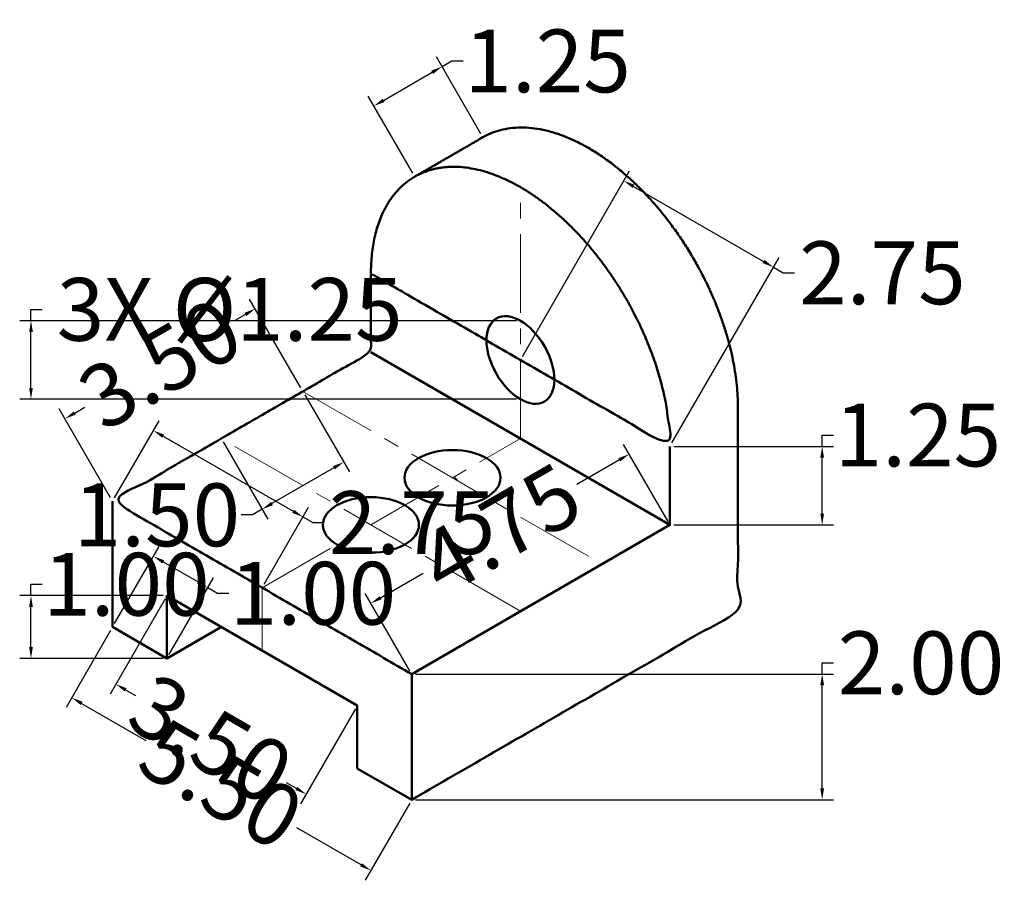
# Model space of a CAD drawing. Units: millimetres. Extents: x 26.3 to 41.9, y 5 to 18.7.
import ezdxf

# ---------------------------------------------------------------- set-up
doc = ezdxf.new("R2010")
doc.units = ezdxf.units.MM
doc.header["$MEASUREMENT"] = 0
doc.linetypes.add('CENTER', pattern=[2, 1.25, -0.25, 0.25, -0.25])
for name, color, linetype, lineweight in [('M-CNTR', 1, 'CENTER', 18), ('M-DIMS', 2, 'Continuous', 25), ('M-OUTL', 7, 'Continuous', 50)]:
    doc.layers.add(name, color=color, linetype=linetype, lineweight=lineweight)
doc.styles.get("Standard").update_dxf_attribs({"font": 'arial.ttf'})
doc.dimstyles.get("Standard").update_dxf_attribs({"dimtxt": 1, "dimasz": 0.18, "dimexe": 0.18, "dimexo": 0.0625, "dimgap": 0.09, "dimtad": 0, "dimtoh": 1, "dimzin": 0, "dimdsep": 46, "dimtxsty": 'Standard', "dimcen": 0.09, "dimadec": 0, "dimazin": 0, "dimtfac": 1, "dimtofl": 0, "dimtmove": 0, "dimatfit": 3, "dimfxl": 1, "dimtolj": 1, "dimtzin": 0, "dimarcsym": 0})

# ---------------------------------------------------------------- blocks, each defined once
blk = doc.blocks.new('*D1')
at = {"layer": 'Defpoints', "color": 0, "transparency": 16777216}
for p in [(28.598, 9.502), (31.629, 7.752), (30.815, 6.341)]:
    blk.add_point(p, dxfattribs=at)
at = {"layer": 'M-DIMS', "color": 0, "lineweight": -2, "transparency": 16777216}
for p, q in [((28.567, 9.448), (27.694, 7.935)), ((27.939, 8.001), (28.098, 7.909)), ((31.598, 7.698), (30.725, 6.185)), ((30.659, 6.431), (30.5, 6.522))]:
    blk.add_line(p, q, dxfattribs=at)
at = {"layer": 'M-DIMS', "color": 0, "transparency": 16777216}
for points in [[(27.954, 8.027), (27.924, 7.975), (27.784, 8.091)], [(30.674, 6.457), (30.644, 6.405), (30.815, 6.341)]]:
    blk.add_solid(points, dxfattribs=at)
at = {"layer": 'M-DIMS', "color": 0, "transparency": 16777216, "insert": (29.299, 7.216), "char_height": 1, "attachment_point": 5, "rotation": 330}
blk.add_mtext('\\A1;3.50', dxfattribs=at)
blk = doc.blocks.new('*D2')
at = {"layer": 'Defpoints', "color": 0, "transparency": 16777216}
for p in [(30.004, 14.067), (30.763, 12.752), (27.732, 11.002)]:
    blk.add_point(p, dxfattribs=at)
at = {"layer": 'M-DIMS', "color": 0, "lineweight": -2, "transparency": 16777216}
for p, q in [((30.732, 12.806), (29.914, 14.222)), ((29.848, 13.977), (29.69, 13.885)), ((27.701, 11.056), (26.883, 12.472)), ((27.129, 12.407), (27.288, 12.498))]:
    blk.add_line(p, q, dxfattribs=at)
at = {"layer": 'M-DIMS', "color": 0, "transparency": 16777216}
for points in [[(29.833, 14.003), (29.863, 13.951), (30.004, 14.067)], [(27.114, 12.433), (27.144, 12.381), (26.973, 12.317)]]:
    blk.add_solid(points, dxfattribs=at)
at = {"layer": 'M-DIMS', "color": 0, "transparency": 16777216, "insert": (28.489, 13.192), "char_height": 1, "attachment_point": 5, "rotation": 30}
blk.add_mtext('\\A1;3.50', dxfattribs=at)
blk = doc.blocks.new('*D3')
at = {"layer": 'Defpoints', "color": 0, "transparency": 16777216}
for p in [(38.256, 14.729), (34.227, 13.252), (36.609, 11.877)]:
    blk.add_point(p, dxfattribs=at)
at = {"layer": 'M-DIMS', "color": 0, "lineweight": -2, "transparency": 16777216}
for p, q in [((34.259, 13.306), (35.964, 16.26)), ((36.03, 16.014), (38.1, 14.819)), ((36.64, 11.931), (38.346, 14.885)), ((38.256, 14.729), (38.412, 14.639)), ((38.412, 14.639), (38.592, 14.639))]:
    blk.add_line(p, q, dxfattribs=at)
at = {"layer": 'M-DIMS', "color": 0, "transparency": 16777216}
for points in [[(36.045, 16.04), (36.015, 15.988), (35.874, 16.104)], [(38.115, 14.845), (38.085, 14.793), (38.256, 14.729)]]:
    blk.add_solid(points, dxfattribs=at)
at = {"layer": 'M-DIMS', "color": 0, "transparency": 16777216, "insert": (39.993, 14.639), "char_height": 1, "attachment_point": 5}
blk.add_mtext('\\A1;2.75', dxfattribs=at)
blk = doc.blocks.new('HOLE-ISO-1_25')
blk.add_ellipse((0.766, 0.442), major_axis=(-0.765, 0), ratio=0.57735)
blk = doc.blocks.new('*D5')
at = {"layer": 'Defpoints', "color": 0, "transparency": 16777216}
for p in [(27.732, 9.002), (27.082, 7.876), (32.495, 6.252)]:
    blk.add_point(p, dxfattribs=at)
at = {"layer": 'M-DIMS', "color": 0, "lineweight": -2, "transparency": 16777216}
for p, q in [((27.701, 8.948), (26.992, 7.72)), ((27.238, 7.786), (28.262, 7.194)), ((32.464, 6.198), (31.755, 4.97)), ((31.689, 5.216), (30.665, 5.807))]:
    blk.add_line(p, q, dxfattribs=at)
at = {"layer": 'M-DIMS', "color": 0, "transparency": 16777216}
for points in [[(27.253, 7.812), (27.223, 7.76), (27.082, 7.876)], [(31.704, 5.242), (31.674, 5.19), (31.845, 5.126)]]:
    blk.add_solid(points, dxfattribs=at)
at = {"layer": 'M-DIMS', "color": 0, "transparency": 16777216, "insert": (29.464, 6.501), "char_height": 1, "attachment_point": 5, "rotation": 330}
blk.add_mtext('\\A1;5.50', dxfattribs=at)
blk = doc.blocks.new('*D6')
at = {"layer": 'Defpoints', "color": 0, "transparency": 16777216}
for p in [(35.959, 11.753), (36.609, 10.627), (32.495, 8.252)]:
    blk.add_point(p, dxfattribs=at)
at = {"layer": 'M-DIMS', "color": 0, "lineweight": -2, "transparency": 16777216}
for p, q in [((36.578, 10.681), (35.869, 11.908)), ((35.803, 11.663), (35.125, 11.271)), ((32.001, 9.468), (32.679, 9.859)), ((32.464, 8.306), (31.755, 9.533))]:
    blk.add_line(p, q, dxfattribs=at)
at = {"layer": 'M-DIMS', "color": 0, "transparency": 16777216}
for points in [[(35.788, 11.689), (35.818, 11.637), (35.959, 11.753)], [(31.986, 9.494), (32.016, 9.442), (31.845, 9.378)]]:
    blk.add_solid(points, dxfattribs=at)
at = {"layer": 'M-DIMS', "color": 0, "transparency": 16777216, "insert": (33.902, 10.565), "char_height": 1, "attachment_point": 5, "rotation": 30}
blk.add_mtext('\\A1;4.75', dxfattribs=at)
blk = doc.blocks.new('*D7')
at = {"layer": 'Defpoints', "color": 0, "transparency": 16777216}
for p in [(36.609, 11.877), (39.033, 11.877), (36.609, 10.627)]:
    blk.add_point(p, dxfattribs=at)
at = {"layer": 'M-DIMS', "color": 0, "lineweight": -2, "transparency": 16777216}
for p, q in [((39.033, 11.877), (39.033, 12.057)), ((39.033, 12.057), (39.213, 12.057)), ((36.671, 11.877), (39.213, 11.877)), ((39.033, 10.807), (39.033, 11.697)), ((36.671, 10.627), (39.213, 10.627))]:
    blk.add_line(p, q, dxfattribs=at)
at = {"layer": 'M-DIMS', "color": 0, "transparency": 16777216}
for points in [[(39.003, 11.697), (39.063, 11.697), (39.033, 11.877)], [(39.003, 10.807), (39.063, 10.807), (39.033, 10.627)]]:
    blk.add_solid(points, dxfattribs=at)
at = {"layer": 'M-DIMS', "color": 0, "transparency": 16777216, "insert": (40.558, 12.057), "char_height": 1, "attachment_point": 5}
blk.add_mtext('\\A1;1.25', dxfattribs=at)
blk = doc.blocks.new('*D8')
at = {"layer": 'Defpoints', "color": 0, "transparency": 16777216}
for p in [(32.979, 17.921), (33.629, 16.795), (32.543, 16.169)]:
    blk.add_point(p, dxfattribs=at)
at = {"layer": 'M-DIMS', "color": 0, "lineweight": -2, "transparency": 16777216}
for p, q in [((33.598, 16.85), (32.889, 18.077)), ((32.979, 17.921), (33.135, 18.011)), ((33.135, 18.011), (33.315, 18.011)), ((32.049, 17.384), (32.823, 17.831)), ((32.512, 16.223), (31.803, 17.45))]:
    blk.add_line(p, q, dxfattribs=at)
at = {"layer": 'M-DIMS', "color": 0, "transparency": 16777216}
for points in [[(32.808, 17.857), (32.838, 17.805), (32.979, 17.921)], [(32.034, 17.41), (32.064, 17.358), (31.893, 17.294)]]:
    blk.add_solid(points, dxfattribs=at)
at = {"layer": 'M-DIMS', "color": 0, "transparency": 16777216, "insert": (34.66, 18.011), "char_height": 1, "attachment_point": 5}
blk.add_mtext('\\A1;1.25', dxfattribs=at)
blk = doc.blocks.new('*D9')
at = {"layer": 'Defpoints', "color": 0, "transparency": 16777216}
for p in [(32.495, 8.252), (39.033, 8.252), (32.495, 6.252)]:
    blk.add_point(p, dxfattribs=at)
at = {"layer": 'M-DIMS', "color": 0, "lineweight": -2, "transparency": 16777216}
for p, q in [((39.033, 8.252), (39.033, 8.432)), ((39.033, 8.432), (39.213, 8.432)), ((32.558, 8.252), (39.213, 8.252)), ((39.033, 6.432), (39.033, 8.072)), ((32.558, 6.252), (39.213, 6.252))]:
    blk.add_line(p, q, dxfattribs=at)
at = {"layer": 'M-DIMS', "color": 0, "transparency": 16777216}
for points in [[(39.003, 8.072), (39.063, 8.072), (39.033, 8.252)], [(39.003, 6.432), (39.063, 6.432), (39.033, 6.252)]]:
    blk.add_solid(points, dxfattribs=at)
at = {"layer": 'M-DIMS', "color": 0, "transparency": 16777216, "insert": (40.608, 8.432), "char_height": 1, "attachment_point": 5}
blk.add_mtext('\\A1;2.00', dxfattribs=at)
blk = doc.blocks.new('*D10')
at = {"layer": 'Defpoints', "color": 0, "transparency": 16777216}
for p in [(26.432139, 9.501761), (28.598164, 9.501761), (28.598164, 8.501761)]:
    blk.add_point(p, dxfattribs=at)
at = {"layer": 'M-DIMS', "color": 0, "lineweight": -2, "transparency": 16777216}
for p, q in [((26.432139, 9.501761), (26.432139, 9.681761)), ((26.432139, 9.681761), (26.612139, 9.681761)), ((28.535664, 9.501761), (26.252139, 9.501761)), ((26.432139, 8.681761), (26.432139, 9.321761)), ((28.535664, 8.501761), (26.252139, 8.501761))]:
    blk.add_line(p, q, dxfattribs=at)
at = {"layer": 'M-DIMS', "color": 0, "transparency": 16777216}
for points in [[(26.402139, 9.321761), (26.462139, 9.321761), (26.432139, 9.501761)], [(26.402139, 8.681761), (26.462139, 8.681761), (26.432139, 8.501761)]]:
    blk.add_solid(points, dxfattribs=at)
at = {"layer": 'M-DIMS', "color": 0, "transparency": 16777216, "insert": (27.952139, 9.681761), "char_height": 1, "attachment_point": 5}
blk.add_mtext('\\A1;1.00', dxfattribs=at)
blk = doc.blocks.new('*D11')
at = {"layer": 'Defpoints', "color": 0, "transparency": 16777216}
for p in [(29.248, 9.628), (27.732, 9.002), (28.598, 8.502)]:
    blk.add_point(p, dxfattribs=at)
at = {"layer": 'M-DIMS', "color": 0, "lineweight": -2, "transparency": 16777216}
for p, q in [((27.763, 9.056), (28.472, 10.283)), ((28.538, 10.038), (29.092, 9.718)), ((28.629, 8.556), (29.338, 9.783)), ((29.248, 9.628), (29.404, 9.538)), ((29.404, 9.538), (29.584, 9.538))]:
    blk.add_line(p, q, dxfattribs=at)
at = {"layer": 'M-DIMS', "color": 0, "transparency": 16777216}
for points in [[(28.553, 10.064), (28.523, 10.012), (28.382, 10.128)], [(29.107, 9.744), (29.077, 9.692), (29.248, 9.628)]]:
    blk.add_solid(points, dxfattribs=at)
at = {"layer": 'M-DIMS', "color": 0, "transparency": 16777216, "insert": (30.924, 9.538), "char_height": 1, "attachment_point": 5}
blk.add_mtext('\\A1;1.00', dxfattribs=at)
blk = doc.blocks.new('*D12')
at = {"layer": 'Defpoints', "color": 0, "transparency": 16777216}
for p in [(30.763, 12.752), (29.464, 12.002), (30.114, 10.876)]:
    blk.add_point(p, dxfattribs=at)
at = {"layer": 'M-DIMS', "color": 0, "lineweight": -2, "transparency": 16777216}
for p, q in [((30.794, 12.698), (31.503, 11.47)), ((29.495, 11.948), (30.204, 10.72)), ((31.257, 11.536), (30.27, 10.966)), ((30.114, 10.876), (29.958, 10.786)), ((29.958, 10.786), (29.778, 10.786))]:
    blk.add_line(p, q, dxfattribs=at)
at = {"layer": 'M-DIMS', "color": 0, "transparency": 16777216}
for points in [[(31.242, 11.562), (31.272, 11.51), (31.413, 11.626)], [(30.255, 10.992), (30.285, 10.94), (30.114, 10.876)]]:
    blk.add_solid(points, dxfattribs=at)
at = {"layer": 'M-DIMS', "color": 0, "transparency": 16777216, "insert": (28.438, 10.786), "char_height": 1, "attachment_point": 5}
blk.add_mtext('\\A1;1.50', dxfattribs=at)
blk = doc.blocks.new('*D13')
at = {"layer": 'Defpoints', "color": 0, "transparency": 16777216}
for p in [(27.732, 11.002), (30.764, 10.753), (30.114, 9.627)]:
    blk.add_point(p, dxfattribs=at)
at = {"layer": 'M-DIMS', "color": 0, "lineweight": -2, "transparency": 16777216}
for p, q in [((27.763, 11.056), (28.472, 12.283)), ((28.538, 12.038), (30.608, 10.843)), ((30.145, 9.681), (30.854, 10.908)), ((30.764, 10.753), (30.92, 10.663)), ((30.92, 10.663), (31.1, 10.663))]:
    blk.add_line(p, q, dxfattribs=at)
at = {"layer": 'M-DIMS', "color": 0, "transparency": 16777216}
for points in [[(28.553, 12.064), (28.523, 12.012), (28.382, 12.128)], [(30.623, 10.869), (30.593, 10.817), (30.764, 10.753)]]:
    blk.add_solid(points, dxfattribs=at)
at = {"layer": 'M-DIMS', "color": 0, "transparency": 16777216, "insert": (32.501, 10.663), "char_height": 1, "attachment_point": 5}
blk.add_mtext('\\A1;2.75', dxfattribs=at)
blk = doc.blocks.new('*D14')
at = {"layer": 'Defpoints', "color": 0, "transparency": 16777216}
for p in [(26.432, 13.877), (34.227, 13.877), (34.227, 12.627)]:
    blk.add_point(p, dxfattribs=at)
at = {"layer": 'M-DIMS', "color": 0, "lineweight": -2, "transparency": 16777216}
for p, q in [((26.432, 13.877), (26.432, 14.057)), ((26.432, 14.057), (26.612, 14.057)), ((34.165, 13.877), (26.252, 13.877)), ((26.432, 12.807), (26.432, 13.697)), ((34.165, 12.627), (26.252, 12.627))]:
    blk.add_line(p, q, dxfattribs=at)
at = {"layer": 'M-DIMS', "color": 0, "transparency": 16777216}
for points in [[(26.402, 13.697), (26.462, 13.697), (26.432, 13.877)], [(26.402, 12.807), (26.462, 12.807), (26.432, 12.627)]]:
    blk.add_solid(points, dxfattribs=at)
at = {"layer": 'M-DIMS', "color": 0, "transparency": 16777216, "insert": (29.596, 14.057), "char_height": 1, "attachment_point": 5}
blk.add_mtext('\\A1;3X %%c1.25', dxfattribs=at)

msp = doc.modelspace()

# ---------------------------------------------------------------- linework, layer by layer
at = {"layer": 'M-CNTR'}
for points in [[(30.114, 8.627), (30.114, 9.627), (34.227, 12.002), (34.227, 16.002)], [(34.227, 9.252), (29.464, 12.002), (29.789, 12.189), (30.763, 12.752), (35.526, 10.002)]]:
    msp.add_lwpolyline(points, dxfattribs=at)
msp.add_ellipse((34.227, 13.252), major_axis=(1.684, -2.917), ratio=0.57735, start_param=5.039609, end_param=5.068087, dxfattribs=at)
at = {"layer": 'M-OUTL'}
for points in [[(36.609, 11.877), (36.609, 10.627), (31.846, 13.377)], [(27.732, 11.002), (27.732, 9.002), (28.598, 8.502), (29.464, 9.002)], [(28.598, 8.502), (28.598, 9.502), (31.629, 7.752), (31.629, 6.752), (32.495, 6.252), (32.495, 8.252), (36.609, 10.627)]]:
    msp.add_lwpolyline(points, dxfattribs=at)
for points, weights, knots in [([(32.495, 6.252), (35.093, 7.752), (37.691, 9.252), (37.691, 10.877), (37.691, 12.502), (37.691, 14.339), (36.221, 15.891), (34.751, 17.443), (33.626, 16.794), (33.085, 16.481), (32.543, 16.169)], [1, 1, 1, 1, 1, 0.831469612303, 1, 0.831469612303, 1, 1, 1], [0, 0, 0, 1, 1, 2, 2, 3.178097, 3.178097, 4.356194, 4.356194, 5.356194, 5.356194, 5.356194]), ([(32.495, 8.252), (30.114, 9.627), (27.732, 11.002), (29.789, 12.189), (31.846, 13.377), (31.846, 14.002), (31.846, 14.627), (34.227, 13.252), (36.609, 11.877), (36.609, 13.464), (35.418, 14.946), (34.227, 16.427), (33.037, 16.321), (31.846, 16.214), (31.846, 14.627)], [1, 1, 1, 1, 1, 1, 1, 1, 1, 0.866025403784, 1, 0.866025403784, 1, 0.866025403784, 1], [0, 0, 0, 1, 1, 2, 2, 3, 3, 4, 4, 5.047198, 5.047198, 6.094395, 6.094395, 7.141593, 7.141593, 7.141593])]:
    msp.add_rational_spline(points, weights, degree=2, knots=knots, dxfattribs=at)

# ---------------------------------------------------------------- block references
at = {"layer": 'M-OUTL', "rotation": 119.9999999999999}
msp.add_blockref('HOLE-ISO-1_25', (34.993, 12.809), dxfattribs=at)
at = {"layer": 'M-OUTL'}
for p in [(32.379, 10.935), (31.08, 10.185)]:
    msp.add_blockref('HOLE-ISO-1_25', p, dxfattribs=at)

# ---------------------------------------------------------------- dimensions: what is measured, and where the dimension line sits
at = {"layer": 'M-DIMS'}
for base, p1, p2, angle, picture, middle in [((32.979, 17.921), (32.543, 16.169), (33.629, 16.795), 29.9997, '*D8', (34.66, 18.011)), ((30.114, 10.876), (30.763, 12.752), (29.464, 12.002), 210, '*D12', (28.438, 10.786)), ((39.033, 11.877), (36.609, 10.627), (36.609, 11.877), 90, '*D7', (40.558, 12.057)), ((30.764, 10.753), (27.732, 11.002), (30.114, 9.627), 330, '*D13', (32.501, 10.663)), ((35.959, 11.753), (32.495, 8.252), (36.609, 10.627), 30, '*D6', (33.902, 10.565)), ((26.432, 9.502), (28.598, 8.502), (28.598, 9.502), 90, '*D10', (27.952, 9.682)), ((29.248, 9.628), (27.732, 9.002), (28.598, 8.502), 330, '*D11', (30.924, 9.538)), ((27.082, 7.876), (32.495, 6.252), (27.732, 9.002), 150, '*D5', (29.464, 6.501)), ((39.033, 8.252), (32.495, 6.252), (32.495, 8.252), 90, '*D9', (40.608, 8.432))]:
    dim = msp.add_linear_dim(base=base, p1=p1, p2=p2, angle=angle, dimstyle='Standard', override={"dimdec": 2, "dimlfac": 1, "dimrnd": 0, "dimzin": 0, "dimdsep": 46, "dimlunit": 2}, dxfattribs=at)
    dim.commit()
    dim.dimension.update_dxf_attribs({"geometry": picture, "text_midpoint": middle})
for p1, p2, distance, picture, middle in [((34.227, 13.252), (36.609, 11.877), 3.294, '*D3', (39.993, 14.639)), ((27.732, 11.002), (30.763, 12.752), 1.518, '*D2', (28.489, 13.192)), ((28.598, 9.502), (31.629, 7.752), -1.629, '*D1', (29.299, 7.216))]:
    dim = msp.add_aligned_dim(p1=p1, p2=p2, distance=distance, dimstyle='Standard', override={"dimclrd": 0, "dimclre": 0, "dimclrt": 0}, dxfattribs=at)
    dim.commit()
    dim.dimension.update_dxf_attribs({"geometry": picture, "text_midpoint": middle})
dim = msp.add_linear_dim(base=(26.432, 13.877), p1=(34.227, 12.627), p2=(34.227, 13.877), angle=90, text='3X %%c<>', dimstyle='Standard', override={"dimdec": 2, "dimlfac": 1, "dimrnd": 0, "dimzin": 0, "dimdsep": 46, "dimlunit": 2}, dxfattribs=at)
dim.commit()
dim.dimension.update_dxf_attribs({"geometry": '*D14', "text_midpoint": (29.596, 14.057)})

doc.saveas('drawing.dxf')
